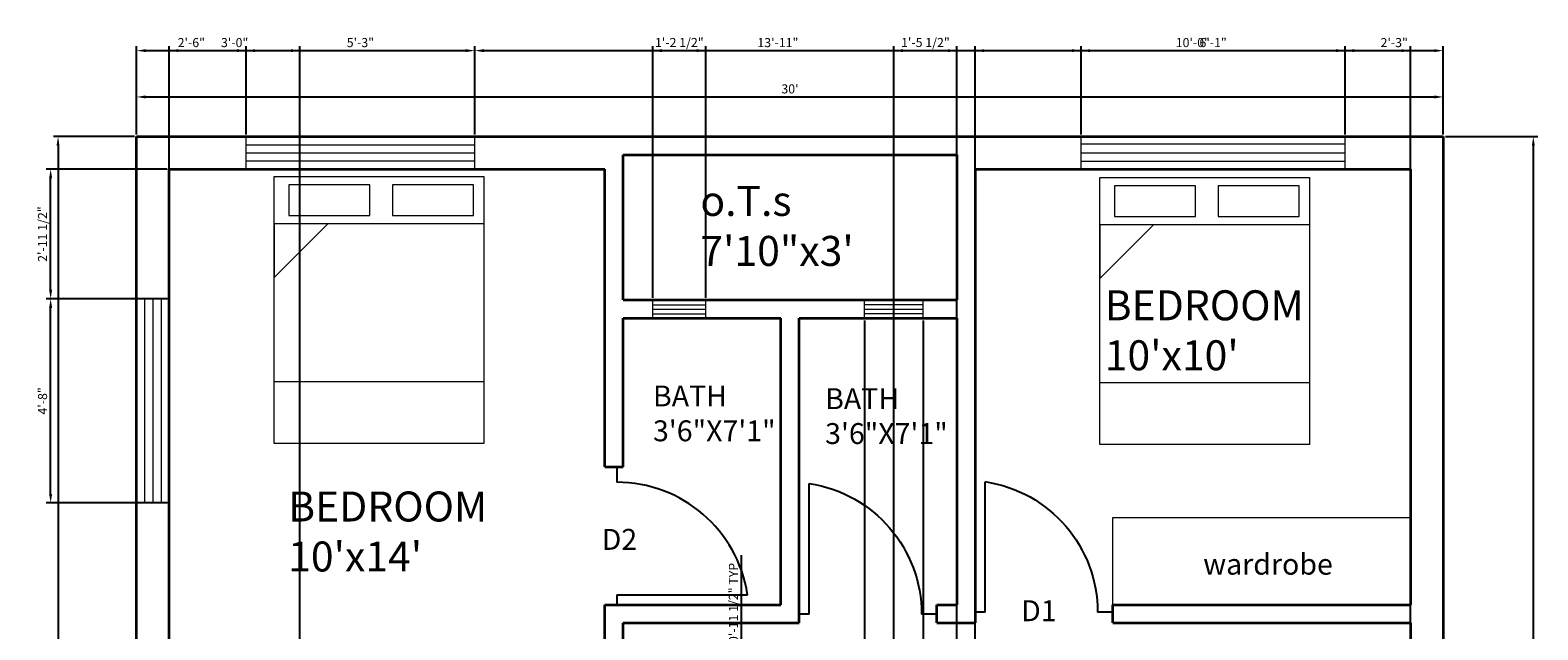
# Model space of a CAD drawing. Units: inches. Extents: x 346 to 762, y 179 to 666.
# Tile 3 of 3: x 346 to 762, y 500 to 666. Entities that reach past the tile are written whole.
import ezdxf

# ---------------------------------------------------------------- set-up
doc = ezdxf.new("R2010")
doc.units = ezdxf.units.IN
for name, color, linetype, lineweight in [('A-ANNO-DIMS', 2, 'Continuous', 18), ('A-ANNO-TEXT', 7, 'Continuous', 18), ('A-AREA-IDEN', 7, 'Continuous', 25), ('A-DOOR', 3, 'Continuous', 25), ('A-FLOR-CASE', 9, 'Continuous', 18), ('A-FURN', 8, 'Continuous', 18), ('A-GLAZ', 4, 'Continuous', 18), ('A-WALL', 7, 'Continuous', 35)]:
    doc.layers.add(name, color=color, linetype=linetype, lineweight=lineweight)
doc.styles.get("Standard").update_dxf_attribs({"font": 'arial.ttf'})
doc.dimstyles.new('ISO-25', dxfattribs={"dimtxt": 2.5, "dimasz": 2.5, "dimexe": 1.25, "dimexo": 0.625, "dimtad": 1, "dimdec": 0, "dimlunit": 3, "dimtxsty": 'Standard', "dimcen": 2.5, "dimadec": 0, "dimazin": 0, "dimtfac": 1, "dimtdec": 0, "dimtmove": 0, "dimatfit": 3, "dimfxl": 1, "dimarcsym": 0})

# ---------------------------------------------------------------- blocks, each defined once
blk = doc.blocks.new('*D1')
at = {"layer": 'A-ANNO-DIMS', "color": 0, "lineweight": -2, "transparency": 16777216}
for p, q in [((375.66, 636.85), (375.66, 648.41)), ((735.66, 636.85), (735.66, 648.41)), ((378.16, 647.16), (733.16, 647.16))]:
    blk.add_line(p, q, dxfattribs=at)
at = {"layer": 'A-ANNO-DIMS', "color": 0, "transparency": 16777216}
for points in [[(378.16, 647.58), (378.16, 646.74), (375.66, 647.16)], [(733.16, 647.58), (733.16, 646.74), (735.66, 647.16)]]:
    blk.add_solid(points, dxfattribs=at)
at = {"layer": 'Defpoints', "color": 0, "transparency": 16777216}
for p in [(735.66, 647.16), (375.66, 636.22), (735.66, 636.22)]:
    blk.add_point(p, dxfattribs=at)
at = {"layer": 'A-ANNO-DIMS', "color": 0, "transparency": 16777216, "insert": (555.66, 649.06), "char_height": 2.5, "attachment_point": 5}
blk.add_mtext("30'", dxfattribs=at)
blk = doc.blocks.new('*D2')
at = {"layer": 'A-ANNO-DIMS', "color": 0, "lineweight": -2, "transparency": 16777216}
for p, q in [((375.04, 636.22), (352.75, 636.22)), ((354, 633.72), (354, 206.72)), ((375.04, 204.22), (352.75, 204.22))]:
    blk.add_line(p, q, dxfattribs=at)
at = {"layer": 'A-ANNO-DIMS', "color": 0, "transparency": 16777216}
for points in [[(353.58, 633.72), (354.41, 633.72), (354, 636.22)], [(353.58, 206.72), (354.41, 206.72), (354, 204.22)]]:
    blk.add_solid(points, dxfattribs=at)
at = {"layer": 'Defpoints', "color": 0, "transparency": 16777216}
for p in [(375.66, 636.22), (354, 204.22), (375.66, 204.22)]:
    blk.add_point(p, dxfattribs=at)
at = {"layer": 'A-ANNO-DIMS', "color": 0, "transparency": 16777216, "insert": (352.1, 420.22), "char_height": 2.5, "attachment_point": 5, "rotation": 90}
blk.add_mtext("36'", dxfattribs=at)
blk = doc.blocks.new('*D3')
at = {"layer": 'A-ANNO-DIMS', "color": 0, "lineweight": -2, "transparency": 16777216}
for p, q in [((736.29, 636.22), (761.72, 636.22)), ((760.47, 633.72), (760.47, 206.72)), ((736.29, 204.22), (761.72, 204.22))]:
    blk.add_line(p, q, dxfattribs=at)
at = {"layer": 'A-ANNO-DIMS', "color": 0, "transparency": 16777216}
for points in [[(760.06, 633.72), (760.89, 633.72), (760.47, 636.22)], [(760.06, 206.72), (760.89, 206.72), (760.47, 204.22)]]:
    blk.add_solid(points, dxfattribs=at)
at = {"layer": 'Defpoints', "color": 0, "transparency": 16777216}
for p in [(735.66, 636.22), (735.66, 204.22), (760.47, 204.22)]:
    blk.add_point(p, dxfattribs=at)
at = {"layer": 'A-ANNO-DIMS', "color": 0, "transparency": 16777216, "insert": (758.57, 420.22), "char_height": 2.5, "attachment_point": 5, "rotation": 90}
blk.add_mtext("36'", dxfattribs=at)
blk = doc.blocks.new('BED-DOUBLE')
for p, q in [((0, 0), (0, 73.56)), ((0, 73.56), (57.79, 73.56)), ((57.79, 73.56), (57.79, 0)), ((0, 56.59), (57.79, 56.59)), ((57.79, 27.81), (42.96, 13.04)), ((57.79, 13.04), (57.79, 27.81)), ((0, 0), (0, 13.04)), ((0, 13.04), (57.79, 13.04)), ((57.79, 0), (0, 0))]:
    blk.add_line(p, q)
for points in [[(2.87, 2.28), (25.15, 2.28), (25.15, 10.76), (2.87, 10.76)], [(31.41, 2.28), (53.7, 2.28), (53.7, 10.76), (31.41, 10.76)]]:
    blk.add_lwpolyline(points, close=True)
blk = doc.blocks.new('DOOR-SINGLE-36IN')
for p, q in [((2.79, 36), (0, 36)), ((2.79, 36), (2.79, 0)), ((38, 36), (33.78, 36))]:
    blk.add_line(p, q)
blk.add_arc((-2.63, 36), 36.41, 278.5676, 0)
blk = doc.blocks.new('*D13')
at = {"layer": 'A-ANNO-DIMS', "color": 0, "lineweight": -2, "transparency": 16777216}
for p, q in [((542.32, 482.35), (542.32, 520.92)), ((543.4, 482.35), (541.07, 482.35)), ((542.32, 473.46), (542.32, 479.85)), ((543.4, 470.96), (541.07, 470.96))]:
    blk.add_line(p, q, dxfattribs=at)
at = {"layer": 'A-ANNO-DIMS', "color": 0, "transparency": 16777216}
for points in [[(541.9, 479.85), (542.74, 479.85), (542.32, 482.35)], [(541.9, 473.46), (542.74, 473.46), (542.32, 470.96)]]:
    blk.add_solid(points, dxfattribs=at)
at = {"layer": 'Defpoints', "color": 0, "transparency": 16777216}
for p in [(542.32, 482.35), (544.03, 482.35), (544.03, 470.96)]:
    blk.add_point(p, dxfattribs=at)
at = {"layer": 'A-ANNO-DIMS', "color": 0, "transparency": 16777216, "insert": (540.4, 502.88), "char_height": 2.5, "attachment_point": 5, "rotation": 90}
blk.add_mtext('CHAIR 0\'-11 1/2" TYP.', dxfattribs=at)
blk = doc.blocks.new('*D18')
at = {"layer": 'A-ANNO-DIMS', "color": 0, "lineweight": -2, "transparency": 16777216}
for p, q in [((584.3, 357.85), (584.3, 661.17)), ((601.66, 357.85), (601.66, 661.17)), ((586.8, 659.92), (599.16, 659.92))]:
    blk.add_line(p, q, dxfattribs=at)
at = {"layer": 'A-ANNO-DIMS', "color": 0, "transparency": 16777216}
for points in [[(586.8, 660.34), (586.8, 659.51), (584.3, 659.92)], [(599.16, 660.34), (599.16, 659.51), (601.66, 659.92)]]:
    blk.add_solid(points, dxfattribs=at)
at = {"layer": 'Defpoints', "color": 0, "transparency": 16777216}
for p in [(601.66, 659.92), (584.3, 357.22), (601.66, 357.22)]:
    blk.add_point(p, dxfattribs=at)
at = {"layer": 'A-ANNO-DIMS', "color": 0, "transparency": 16777216, "insert": (592.98, 661.84), "char_height": 2.5, "attachment_point": 5}
blk.add_mtext('1\'-5 1/2"', dxfattribs=at)
blk = doc.blocks.new('*D29')
at = {"layer": 'A-ANNO-DIMS', "color": 0, "lineweight": -2, "transparency": 16777216}
for p, q in [((384.66, 362.85), (384.66, 661.17)), ((420.66, 362.85), (420.66, 661.17)), ((387.16, 659.92), (418.16, 659.92))]:
    blk.add_line(p, q, dxfattribs=at)
at = {"layer": 'A-ANNO-DIMS', "color": 0, "transparency": 16777216}
for points in [[(387.16, 660.34), (387.16, 659.51), (384.66, 659.92)], [(418.16, 660.34), (418.16, 659.51), (420.66, 659.92)]]:
    blk.add_solid(points, dxfattribs=at)
at = {"layer": 'Defpoints', "color": 0, "transparency": 16777216}
for p in [(420.66, 659.92), (384.66, 362.22), (420.66, 362.22)]:
    blk.add_point(p, dxfattribs=at)
at = {"layer": 'A-ANNO-DIMS', "color": 0, "transparency": 16777216, "insert": (402.66, 661.82), "char_height": 2.5, "attachment_point": 5}
blk.add_mtext('3\'-0"', dxfattribs=at)
blk = doc.blocks.new('*D30')
at = {"layer": 'A-ANNO-DIMS', "color": 0, "lineweight": -2, "transparency": 16777216}
for p, q in [((375.66, 636.85), (375.66, 661.17)), ((405.8, 636.85), (405.8, 661.17)), ((378.16, 659.92), (403.3, 659.92))]:
    blk.add_line(p, q, dxfattribs=at)
at = {"layer": 'A-ANNO-DIMS', "color": 0, "transparency": 16777216}
for points in [[(378.16, 660.34), (378.16, 659.51), (375.66, 659.92)], [(403.3, 660.34), (403.3, 659.51), (405.8, 659.92)]]:
    blk.add_solid(points, dxfattribs=at)
at = {"layer": 'Defpoints', "color": 0, "transparency": 16777216}
for p in [(405.8, 659.92), (375.66, 636.22), (405.8, 636.22)]:
    blk.add_point(p, dxfattribs=at)
at = {"layer": 'A-ANNO-DIMS', "color": 0, "transparency": 16777216, "insert": (390.73, 661.82), "char_height": 2.5, "attachment_point": 5}
blk.add_mtext('2\'-6"', dxfattribs=at)
blk = doc.blocks.new('*D31')
at = {"layer": 'A-ANNO-DIMS', "color": 0, "lineweight": -2, "transparency": 16777216}
for p, q in [((405.8, 636.85), (405.8, 661.17)), ((468.82, 636.85), (468.82, 661.17)), ((408.3, 659.92), (466.32, 659.92))]:
    blk.add_line(p, q, dxfattribs=at)
at = {"layer": 'A-ANNO-DIMS', "color": 0, "transparency": 16777216}
for points in [[(408.3, 660.34), (408.3, 659.51), (405.8, 659.92)], [(466.32, 660.34), (466.32, 659.51), (468.82, 659.92)]]:
    blk.add_solid(points, dxfattribs=at)
at = {"layer": 'Defpoints', "color": 0, "transparency": 16777216}
for p in [(468.82, 659.92), (405.8, 636.22), (468.82, 636.22)]:
    blk.add_point(p, dxfattribs=at)
at = {"layer": 'A-ANNO-DIMS', "color": 0, "transparency": 16777216, "insert": (437.31, 661.82), "char_height": 2.5, "attachment_point": 5}
blk.add_mtext('5\'-3"', dxfattribs=at)
blk = doc.blocks.new('*D32')
at = {"layer": 'A-ANNO-DIMS', "color": 0, "lineweight": -2, "transparency": 16777216}
for p, q in [((468.82, 636.85), (468.82, 661.17)), ((635.86, 636.85), (635.86, 661.17)), ((471.32, 659.92), (633.36, 659.92))]:
    blk.add_line(p, q, dxfattribs=at)
at = {"layer": 'A-ANNO-DIMS', "color": 0, "transparency": 16777216}
for points in [[(471.32, 660.34), (471.32, 659.51), (468.82, 659.92)], [(633.36, 660.34), (633.36, 659.51), (635.86, 659.92)]]:
    blk.add_solid(points, dxfattribs=at)
at = {"layer": 'Defpoints', "color": 0, "transparency": 16777216}
for p in [(635.86, 659.92), (468.82, 636.22), (635.86, 636.22)]:
    blk.add_point(p, dxfattribs=at)
at = {"layer": 'A-ANNO-DIMS', "color": 0, "transparency": 16777216, "insert": (552.34, 661.82), "char_height": 2.5, "attachment_point": 5}
blk.add_mtext('13\'-11"', dxfattribs=at)
blk = doc.blocks.new('*D33')
at = {"layer": 'A-ANNO-DIMS', "color": 0, "lineweight": -2, "transparency": 16777216}
for p, q in [((635.86, 636.85), (635.86, 661.17)), ((708.64, 636.85), (708.64, 661.17)), ((638.36, 659.92), (706.14, 659.92))]:
    blk.add_line(p, q, dxfattribs=at)
at = {"layer": 'A-ANNO-DIMS', "color": 0, "transparency": 16777216}
for points in [[(638.36, 660.34), (638.36, 659.51), (635.86, 659.92)], [(706.14, 660.34), (706.14, 659.51), (708.64, 659.92)]]:
    blk.add_solid(points, dxfattribs=at)
at = {"layer": 'Defpoints', "color": 0, "transparency": 16777216}
for p in [(708.64, 659.92), (635.86, 636.22), (708.64, 636.22)]:
    blk.add_point(p, dxfattribs=at)
at = {"layer": 'A-ANNO-DIMS', "color": 0, "transparency": 16777216, "insert": (672.25, 661.82), "char_height": 2.5, "attachment_point": 5}
blk.add_mtext('6\'-1"', dxfattribs=at)
blk = doc.blocks.new('*D34')
at = {"layer": 'A-ANNO-DIMS', "color": 0, "lineweight": -2, "transparency": 16777216}
for p, q in [((708.64, 636.85), (708.64, 661.17)), ((735.66, 636.85), (735.66, 661.17)), ((711.14, 659.92), (733.16, 659.92))]:
    blk.add_line(p, q, dxfattribs=at)
at = {"layer": 'A-ANNO-DIMS', "color": 0, "transparency": 16777216}
for points in [[(711.14, 660.34), (711.14, 659.51), (708.64, 659.92)], [(733.16, 660.34), (733.16, 659.51), (735.66, 659.92)]]:
    blk.add_solid(points, dxfattribs=at)
at = {"layer": 'Defpoints', "color": 0, "transparency": 16777216}
for p in [(735.66, 659.92), (708.64, 636.22), (735.66, 636.22)]:
    blk.add_point(p, dxfattribs=at)
at = {"layer": 'A-ANNO-DIMS', "color": 0, "transparency": 16777216, "insert": (722.15, 661.82), "char_height": 2.5, "attachment_point": 5}
blk.add_mtext('2\'-3"', dxfattribs=at)
blk = doc.blocks.new('*D35')
at = {"layer": 'A-ANNO-DIMS', "color": 0, "lineweight": -2, "transparency": 16777216}
for p, q in [((384.04, 591.53), (350.71, 591.53)), ((351.96, 537.79), (351.96, 589.03)), ((384.04, 535.29), (350.71, 535.29))]:
    blk.add_line(p, q, dxfattribs=at)
at = {"layer": 'A-ANNO-DIMS', "color": 0, "transparency": 16777216}
for points in [[(351.54, 589.03), (352.38, 589.03), (351.96, 591.53)], [(351.54, 537.79), (352.38, 537.79), (351.96, 535.29)]]:
    blk.add_solid(points, dxfattribs=at)
at = {"layer": 'Defpoints', "color": 0, "transparency": 16777216}
for p in [(351.96, 591.53), (384.66, 591.53), (384.66, 535.29)]:
    blk.add_point(p, dxfattribs=at)
at = {"layer": 'A-ANNO-DIMS', "color": 0, "transparency": 16777216, "insert": (350.06, 563.41), "char_height": 2.5, "attachment_point": 5, "rotation": 90}
blk.add_mtext('4\'-8"', dxfattribs=at)
blk = doc.blocks.new('*D36')
at = {"layer": 'A-ANNO-DIMS', "color": 0, "lineweight": -2, "transparency": 16777216}
for p, q in [((384.04, 627.22), (350.71, 627.22)), ((351.96, 594.03), (351.96, 624.72)), ((384.04, 591.53), (350.71, 591.53))]:
    blk.add_line(p, q, dxfattribs=at)
at = {"layer": 'A-ANNO-DIMS', "color": 0, "transparency": 16777216}
for points in [[(351.54, 624.72), (352.38, 624.72), (351.96, 627.22)], [(351.54, 594.03), (352.38, 594.03), (351.96, 591.53)]]:
    blk.add_solid(points, dxfattribs=at)
at = {"layer": 'Defpoints', "color": 0, "transparency": 16777216}
for p in [(351.96, 627.22), (384.66, 627.22), (384.66, 591.53)]:
    blk.add_point(p, dxfattribs=at)
at = {"layer": 'A-ANNO-DIMS', "color": 0, "transparency": 16777216, "insert": (350.04, 609.37), "char_height": 2.5, "attachment_point": 5, "rotation": 90}
blk.add_mtext('2\'-11 1/2"', dxfattribs=at)
blk = doc.blocks.new('*D39')
at = {"layer": 'A-ANNO-DIMS', "color": 0, "lineweight": -2, "transparency": 16777216}
for p, q in [((606.66, 209.85), (606.66, 661.17)), ((726.66, 209.85), (726.66, 661.17)), ((609.16, 659.92), (724.16, 659.92))]:
    blk.add_line(p, q, dxfattribs=at)
at = {"layer": 'A-ANNO-DIMS', "color": 0, "transparency": 16777216}
for points in [[(609.16, 660.34), (609.16, 659.51), (606.66, 659.92)], [(724.16, 660.34), (724.16, 659.51), (726.66, 659.92)]]:
    blk.add_solid(points, dxfattribs=at)
at = {"layer": 'Defpoints', "color": 0, "transparency": 16777216}
for p in [(726.66, 659.92), (606.66, 209.22), (726.66, 209.22)]:
    blk.add_point(p, dxfattribs=at)
at = {"layer": 'A-ANNO-DIMS', "color": 0, "transparency": 16777216, "insert": (666.66, 661.82), "char_height": 2.5, "attachment_point": 5}
blk.add_mtext('10\'-0"', dxfattribs=at)
blk = doc.blocks.new('*D45')
at = {"layer": 'A-ANNO-DIMS', "color": 0, "lineweight": -2, "transparency": 16777216}
for p, q in [((517.89, 591.85), (517.89, 661.17)), ((532.47, 591.85), (532.47, 661.17)), ((520.39, 659.92), (529.97, 659.92))]:
    blk.add_line(p, q, dxfattribs=at)
at = {"layer": 'A-ANNO-DIMS', "color": 0, "transparency": 16777216}
for points in [[(520.39, 660.34), (520.39, 659.51), (517.89, 659.92)], [(529.97, 660.34), (529.97, 659.51), (532.47, 659.92)]]:
    blk.add_solid(points, dxfattribs=at)
at = {"layer": 'Defpoints', "color": 0, "transparency": 16777216}
for p in [(532.47, 659.92), (517.89, 591.22), (532.47, 591.22)]:
    blk.add_point(p, dxfattribs=at)
at = {"layer": 'A-ANNO-DIMS', "color": 0, "transparency": 16777216, "insert": (525.18, 661.84), "char_height": 2.5, "attachment_point": 5}
blk.add_mtext('1\'-2 1/2"', dxfattribs=at)
blk = doc.blocks.new('*D46')
at = {"layer": 'A-ANNO-DIMS', "color": 0, "lineweight": -2, "transparency": 16777216}
for p, q in [((576.21, 585.6), (576.21, 179.27)), ((592.38, 585.6), (592.38, 179.27)), ((578.71, 180.52), (589.88, 180.52))]:
    blk.add_line(p, q, dxfattribs=at)
at = {"layer": 'A-ANNO-DIMS', "color": 0, "transparency": 16777216}
for points in [[(578.71, 180.94), (578.71, 180.11), (576.21, 180.52)], [(589.88, 180.94), (589.88, 180.11), (592.38, 180.52)]]:
    blk.add_solid(points, dxfattribs=at)
at = {"layer": 'Defpoints', "color": 0, "transparency": 16777216}
for p in [(576.21, 586.22), (592.38, 586.22), (592.38, 180.52)]:
    blk.add_point(p, dxfattribs=at)
at = {"layer": 'A-ANNO-DIMS', "color": 0, "transparency": 16777216, "insert": (584.3, 182.4), "char_height": 2.5, "attachment_point": 5}
blk.add_mtext('1\'-4"', dxfattribs=at)

msp = doc.modelspace()

# ---------------------------------------------------------------- linework, layer by layer
at = {"layer": 'A-FLOR-CASE'}
for p, q in [((644.66, 507.22), (644.66, 531.27)), ((644.66, 531.27), (726.66, 531.27))]:
    msp.add_line(p, q, dxfattribs=at)
at = {"layer": 'A-GLAZ'}
for p, q in [((405.8, 627.22), (405.8, 636.22)), ((468.82, 627.22), (468.82, 636.22)), ((635.86, 627.22), (635.86, 636.22)), ((708.64, 627.22), (708.64, 636.22)), ((405.8, 634), (468.82, 634)), ((405.8, 631.72), (468.82, 631.72)), ((635.86, 634.25), (708.64, 634.25)), ((635.86, 631.72), (708.64, 631.72)), ((405.8, 629.52), (468.82, 629.52)), ((635.86, 629.48), (708.64, 629.48)), ((384.66, 591.53), (375.66, 591.53)), ((377.83, 591.53), (377.83, 535.29)), ((380.16, 591.53), (380.16, 535.29)), ((382.4, 591.53), (382.4, 535.29)), ((517.89, 586.22), (517.89, 591.22)), ((517.89, 589.89), (532.47, 589.89)), ((532.47, 586.22), (532.47, 591.22)), ((576.21, 586.22), (576.21, 591.22)), ((576.21, 589.95), (592.38, 589.95)), ((592.38, 586.22), (592.38, 591.22)), ((517.89, 588.72), (532.47, 588.72)), ((517.89, 587.39), (532.47, 587.39)), ((576.21, 588.72), (592.38, 588.72)), ((576.21, 587.5), (592.38, 587.5)), ((384.66, 535.29), (375.66, 535.29))]:
    msp.add_line(p, q, dxfattribs=at)
at = {"layer": 'A-WALL'}
for p, q in [((375.66, 204.22), (375.66, 636.22)), ((375.66, 636.22), (735.66, 636.22)), ((735.66, 636.22), (735.66, 204.22)), ((509.66, 591.22), (509.66, 631.22)), ((509.66, 631.22), (601.66, 631.22)), ((601.66, 631.22), (601.66, 591.22)), ((384.66, 627.22), (504.66, 627.22)), ((384.66, 459.22), (384.66, 627.22)), ((504.66, 545.22), (504.66, 627.22)), ((606.66, 627.22), (606.66, 502.22)), ((606.66, 627.22), (726.66, 627.22)), ((726.66, 627.22), (726.66, 507.22)), ((509.66, 591.22), (601.66, 591.22)), ((509.66, 586.22), (553.16, 586.22)), ((509.66, 545.22), (509.66, 586.22)), ((553.16, 507.22), (553.16, 586.22)), ((558.16, 586.22), (601.66, 586.22)), ((558.16, 502.22), (558.16, 586.22)), ((601.66, 586.22), (601.66, 507.22)), ((504.66, 545.22), (509.66, 545.22)), ((504.66, 507.22), (553.16, 507.22)), ((504.66, 497.22), (504.66, 507.22)), ((596.16, 502.22), (596.16, 507.22)), ((596.16, 507.22), (601.66, 507.22)), ((644.66, 502.22), (644.66, 507.22)), ((644.66, 507.22), (726.66, 507.22)), ((509.66, 502.22), (558.16, 502.22)), ((509.66, 497.22), (509.66, 502.22)), ((596.16, 502.22), (606.66, 502.22)), ((644.66, 502.22), (726.66, 502.22)), ((726.66, 502.22), (726.66, 362.22))]:
    msp.add_line(p, q, dxfattribs=at)

# ---------------------------------------------------------------- block references
at = {"layer": 'A-DOOR', "rotation": 90.0000000000015}
msp.add_blockref('DOOR-SINGLE-36IN', (543.94, 507.22), dxfattribs=at)
at = {"layer": 'A-DOOR', "extrusion": (0, 0, -1), "zscale": -1, "rotation": 180}
for p in [(-558.16, 540.65), (-606.66, 541.15)]:
    msp.add_blockref('DOOR-SINGLE-36IN', p, dxfattribs=at)
at = {"layer": 'A-FURN', "rotation": 180}
for p in [(471.3, 625.24), (698.82, 624.99)]:
    msp.add_blockref('BED-DOUBLE', p, dxfattribs=at)

# ---------------------------------------------------------------- texts
at = {"layer": 'A-ANNO-TEXT', "char_height": 5.764, "attachment_point": 1}
for s, insert in [('D2', (503.79, 528.13)), ('wardrobe', (669.53, 521.3)), ('D1', (619.35, 508.47))]:
    msp.add_mtext_dynamic_manual_height_columns(s, width=202.5556, gutter_width=28.82, heights=[0], dxfattribs=dict(at, insert=insert))
at = {"layer": 'A-AREA-IDEN', "attachment_point": 1}
for s, width, gutter_width, insert, char_height in [('o.T.s\\P7\'10"x3\'', 290.4031, 41.32, (530.98, 622.64), 8.263), ("BEDROOM\\P10'x10'", 290.4031, 41.32, (642.39, 593.88), 8.263), ('BATH\\P3\'6"X7\'1"', 202.5556, 28.82, (517.92, 567.65), 5.764), ('BATH\\P3\'6"X7\'1"', 202.5556, 28.82, (565.35, 566.9), 5.764), ("BEDROOM\\P10'x14'", 290.4031, 41.32, (417.41, 538.44), 8.263)]:
    msp.add_mtext_dynamic_manual_height_columns(s, width=width, gutter_width=gutter_width, heights=[0], dxfattribs=dict(at, insert=insert, char_height=char_height))

# ---------------------------------------------------------------- dimensions: what is measured, and where the dimension line sits
at = {"layer": 'A-ANNO-DIMS'}
for base, p1, p2, override, picture, middle in [((532.47, 659.92), (517.89, 591.22), (532.47, 591.22), {"dimdec": 1, "dimlfac": 1, "dimrnd": 0, "dimzin": 1, "dimdsep": 46, "dimlunit": 4, "dimfrac": 2}, '*D45', (525.18, 661.84)), ((601.66, 659.92), (584.3, 357.22), (601.66, 357.22), {"dimdec": 1, "dimlfac": 1, "dimrnd": 0, "dimzin": 1, "dimdsep": 46, "dimlunit": 4, "dimfrac": 2}, '*D18', (592.98, 661.84)), ((405.8, 659.92), (375.66, 636.22), (405.8, 636.22), {"dimdec": 1, "dimlfac": 1, "dimrnd": 0, "dimzin": 1, "dimdsep": 46, "dimlunit": 4, "dimfrac": 2}, '*D30', (390.73, 661.82)), ((420.66, 659.92), (384.66, 362.22), (420.66, 362.22), {"dimdec": 1, "dimlfac": 1, "dimrnd": 0, "dimzin": 1, "dimdsep": 46, "dimlunit": 4, "dimfrac": 2}, '*D29', (402.66, 661.82)), ((468.82, 659.92), (405.8, 636.22), (468.82, 636.22), {"dimdec": 1, "dimlfac": 1, "dimrnd": 0, "dimzin": 1, "dimdsep": 46, "dimlunit": 4, "dimfrac": 2}, '*D31', (437.31, 661.82)), ((635.86, 659.92), (468.82, 636.22), (635.86, 636.22), {"dimdec": 1, "dimlfac": 1, "dimrnd": 0, "dimzin": 1, "dimdsep": 46, "dimlunit": 4, "dimfrac": 2}, '*D32', (552.34, 661.82)), ((726.66, 659.92), (606.66, 209.22), (726.66, 209.22), {"dimdec": 1, "dimlfac": 1, "dimrnd": 0, "dimzin": 1, "dimdsep": 46, "dimlunit": 4, "dimfrac": 2}, '*D39', (666.66, 661.82)), ((708.64, 659.92), (635.86, 636.22), (708.64, 636.22), {"dimdec": 1, "dimlfac": 1, "dimrnd": 0, "dimzin": 1, "dimdsep": 46, "dimlunit": 4, "dimfrac": 2}, '*D33', (672.25, 661.82)), ((735.66, 659.92), (708.64, 636.22), (735.66, 636.22), {"dimdec": 1, "dimlfac": 1, "dimrnd": 0, "dimzin": 1, "dimdsep": 46, "dimlunit": 4, "dimfrac": 2}, '*D34', (722.15, 661.82)), ((735.66, 647.16), (375.66, 636.22), (735.66, 636.22), {"dimclrd": 0, "dimclre": 0, "dimclrt": 0}, '*D1', (555.66, 649.06)), ((592.38, 180.52), (576.21, 586.22), (592.38, 586.22), {"dimdec": 1, "dimlfac": 1, "dimrnd": 0, "dimzin": 1, "dimdsep": 46, "dimlunit": 4, "dimfrac": 2}, '*D46', (584.3, 182.4))]:
    dim = msp.add_linear_dim(base=base, p1=p1, p2=p2, dimstyle='ISO-25', override=override, dxfattribs=at)
    dim.commit()
    dim.dimension.update_dxf_attribs({"geometry": picture, "text_midpoint": middle})
for base, p1, p2, override, picture, middle in [((354, 204.22), (375.66, 636.22), (375.66, 204.22), {"dimclrd": 0, "dimclre": 0, "dimclrt": 0}, '*D2', (352.1, 420.22)), ((760.47, 204.22), (735.66, 636.22), (735.66, 204.22), {"dimclrd": 0, "dimclre": 0, "dimclrt": 0}, '*D3', (758.57, 420.22)), ((351.96, 627.22), (384.66, 591.53), (384.66, 627.22), {"dimdec": 1, "dimlfac": 1, "dimrnd": 0, "dimzin": 1, "dimdsep": 46, "dimlunit": 4, "dimfrac": 2}, '*D36', (350.04, 609.37)), ((351.96, 591.53), (384.66, 535.29), (384.66, 591.53), {"dimdec": 1, "dimlfac": 1, "dimrnd": 0, "dimzin": 1, "dimdsep": 46, "dimlunit": 4, "dimfrac": 2}, '*D35', (350.06, 563.41))]:
    dim = msp.add_linear_dim(base=base, p1=p1, p2=p2, angle=90, dimstyle='ISO-25', override=override, dxfattribs=at)
    dim.commit()
    dim.dimension.update_dxf_attribs({"geometry": picture, "text_midpoint": middle})
dim = msp.add_linear_dim(base=(542.32, 482.35), p1=(544.03, 470.96), p2=(544.03, 482.35), angle=90, text='CHAIR <> TYP.', dimstyle='ISO-25', override={"dimdec": 1, "dimlfac": 1, "dimrnd": 0, "dimzin": 1, "dimdsep": 46, "dimlunit": 4, "dimfrac": 2}, dxfattribs=at)
dim.commit()
dim.dimension.update_dxf_attribs({"geometry": '*D13', "text_midpoint": (540.4, 502.88)})

doc.saveas('drawing.dxf')
